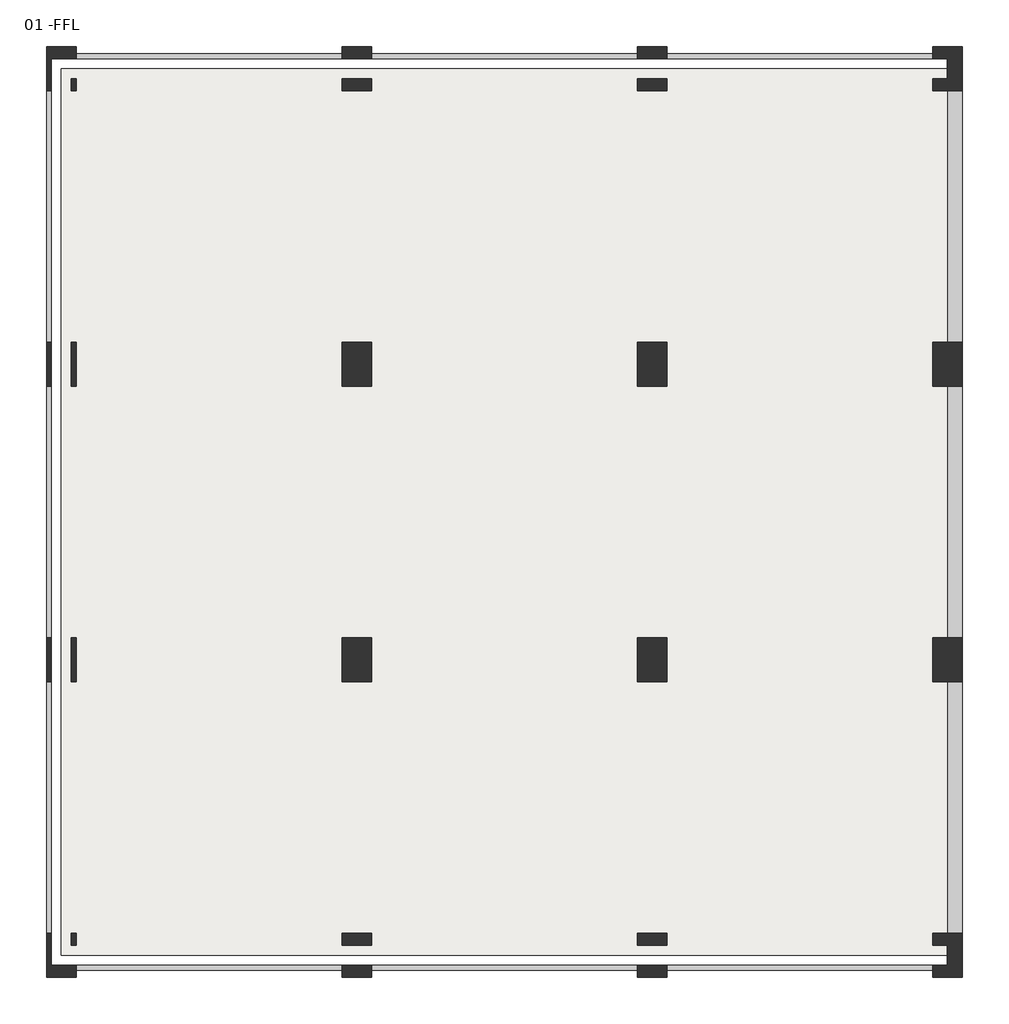
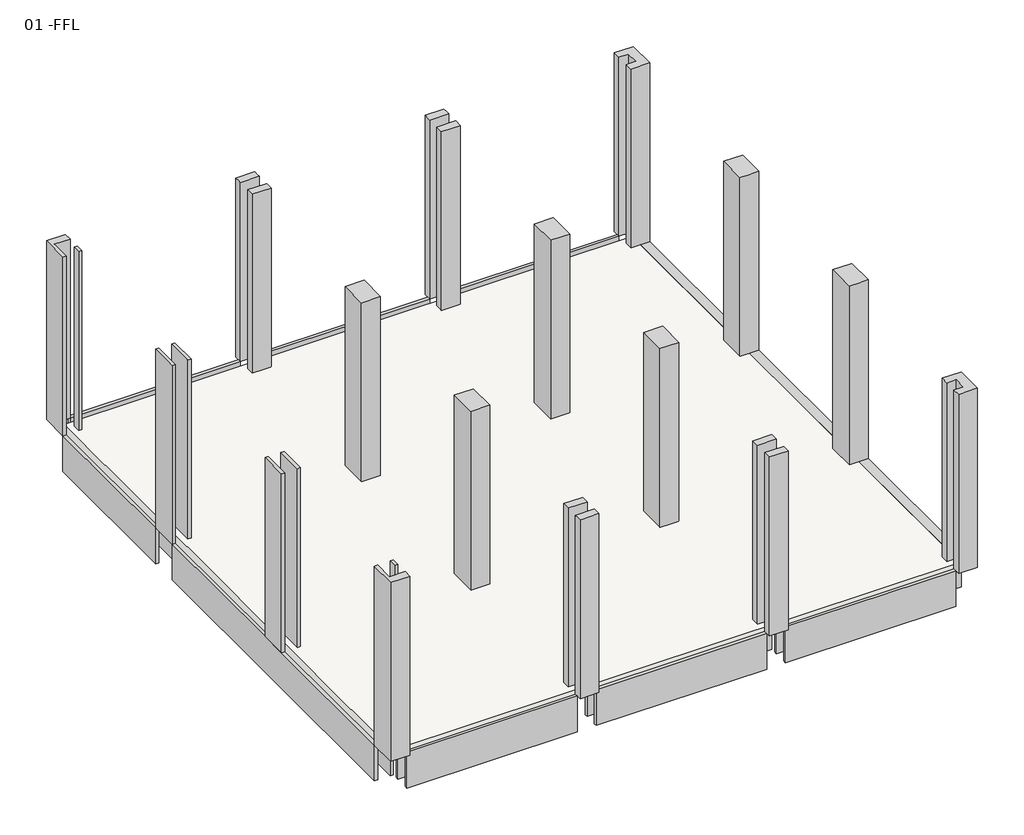
# One storey: 16 columns, 6 beams, 1 slab.
"""IFC4 building model written with IfcOpenShell, lengths in millimetres."""

from ifc_helpers import new_model, si_unit, frame, origin, place, context, project, spatial, polyline, outline, extrude, faceted_brep, element, save

model = new_model("IFC4")

# Units and contexts
model_context = context("Model", 3, world=origin())
ifc_project = project(units=[si_unit("LENGTHUNIT", "METRE", prefix="MILLI")], contexts=[model_context])

# Site, building, storey
site = spatial("IfcSite", under=ifc_project)
building = spatial("IfcBuilding", under=site)
storey = spatial("IfcBuildingStorey", under=building, Name="01 -FFL", Elevation=3048.0)

# Beams
placement = place(None, origin())
element("IfcBeam", 1, ObjectType="Concrete-Rectangular Beam : 12 x 24", at=placement, inside=storey, context=model_context, shape_type="SweptSolid", body=[
    extrude(outline(polyline([(-15593.7609662, 12775.9972109), (-12850.5609662, 12775.9972109), (-12850.5609662, 12725.1972109), (-15593.7609662, 12725.1972109), (-15593.7609662, 12775.9972109)])), frame((0.0, 0.0, 2438.4), z_axis=(0.0, 0.0, 1.0), x_axis=(1.0, 0.0, 0.0)), (0.0, 0.0, 1.0), 609.6),
    extrude(outline(polyline([(-12850.5609662, 12471.1972109), (-15593.7609662, 12471.1972109), (-15593.7609662, 12521.9972109), (-12850.5609662, 12521.9972109), (-12850.5609662, 12471.1972109)])), frame((0.0, 0.0, 2438.4), z_axis=(0.0, 0.0, 1.0), x_axis=(1.0, 0.0, 0.0)), (0.0, 0.0, 1.0), 457.2),
    extrude(outline(polyline([(-18946.5609662, 12471.1972109), (-21689.7609662, 12471.1972109), (-21689.7609662, 12521.9972109), (-18946.5609662, 12521.9972109), (-18946.5609662, 12471.1972109)])), frame((0.0, 0.0, 2438.4), z_axis=(0.0, 0.0, 1.0), x_axis=(1.0, 0.0, 0.0)), (0.0, 0.0, 1.0), 457.2),
    extrude(outline(polyline([(-15898.5609662, 12471.1972109), (-18641.7609662, 12471.1972109), (-18641.7609662, 12521.9972109), (-15898.5609662, 12521.9972109), (-15898.5609662, 12471.1972109)])), frame((0.0, 0.0, 2438.4), z_axis=(0.0, 0.0, 1.0), x_axis=(1.0, 0.0, 0.0)), (0.0, 0.0, 1.0), 457.2),
    extrude(outline(polyline([(-18641.7609662, 12775.9972109), (-15898.5609662, 12775.9972109), (-15898.5609662, 12725.1972109), (-18641.7609662, 12725.1972109), (-18641.7609662, 12775.9972109)])), frame((0.0, 0.0, 2438.4), z_axis=(0.0, 0.0, 1.0), x_axis=(1.0, 0.0, 0.0)), (0.0, 0.0, 1.0), 609.6),
    extrude(outline(polyline([(-21689.7609662, 12775.9972109), (-18946.5609662, 12775.9972109), (-18946.5609662, 12725.1972109), (-21689.7609662, 12725.1972109), (-21689.7609662, 12775.9972109)])), frame((0.0, 0.0, 2438.4), z_axis=(0.0, 0.0, 1.0), x_axis=(1.0, 0.0, 0.0)), (0.0, 0.0, 1.0), 609.6),
])
element("IfcBeam", 2, ObjectType="Concrete-Rectangular Beam : 12 x 24", at=placement, inside=storey, context=model_context, shape_type="SweptSolid", body=[
    extrude(outline(polyline([(2438.4, -12850.5609662), (2438.4, -12545.7609662), (3048.0, -12545.7609662), (3048.0, -12698.1609662), (2895.6, -12698.1609662), (2895.6, -12850.5609662), (2438.4, -12850.5609662)])), frame((0.0, 3708.1972109, 0.0), z_axis=(0.0, 1.0, 0.0), x_axis=(0.0, 0.0, 1.0)), (0.0, 0.0, 1.0), 2590.8),
    extrude(outline(polyline([(2438.4, -12850.5609662), (2438.4, -12545.7609662), (3048.0, -12545.7609662), (3048.0, -12698.1609662), (2895.6, -12698.1609662), (2895.6, -12850.5609662), (2438.4, -12850.5609662)])), frame((0.0, 9804.1972109, 0.0), z_axis=(0.0, 1.0, 0.0), x_axis=(0.0, 0.0, 1.0)), (0.0, 0.0, 1.0), 2590.8),
    extrude(outline(polyline([(2438.4, -12850.5609662), (2438.4, -12545.7609662), (3048.0, -12545.7609662), (3048.0, -12698.1609662), (2895.6, -12698.1609662), (2895.6, -12850.5609662), (2438.4, -12850.5609662)])), frame((0.0, 6756.1972109, 0.0), z_axis=(0.0, 1.0, 0.0), x_axis=(0.0, 0.0, 1.0)), (0.0, 0.0, 1.0), 2590.8),
])
element("IfcBeam", 3, ObjectType="Concrete-Rectangular Beam : 12 x 24", at=placement, inside=storey, context=model_context, shape_type="SweptSolid", body=[
    extrude(outline(polyline([(-18946.5609662, 3327.1972109), (-21689.7609662, 3327.1972109), (-21689.7609662, 3377.9972109), (-18946.5609662, 3377.9972109), (-18946.5609662, 3327.1972109)])), frame((0.0, 0.0, 2438.4), z_axis=(0.0, 0.0, 1.0), x_axis=(1.0, 0.0, 0.0)), (0.0, 0.0, 1.0), 609.6),
    extrude(outline(polyline([(-21689.7609662, 3631.9972109), (-18946.5609662, 3631.9972109), (-18946.5609662, 3581.1972109), (-21689.7609662, 3581.1972109), (-21689.7609662, 3631.9972109)])), frame((0.0, 0.0, 2438.4), z_axis=(0.0, 0.0, 1.0), x_axis=(1.0, 0.0, 0.0)), (0.0, 0.0, 1.0), 457.2),
    extrude(outline(polyline([(-12850.5609662, 3327.1972109), (-15593.7609662, 3327.1972109), (-15593.7609662, 3377.9972109), (-12850.5609662, 3377.9972109), (-12850.5609662, 3327.1972109)])), frame((0.0, 0.0, 2438.4), z_axis=(0.0, 0.0, 1.0), x_axis=(1.0, 0.0, 0.0)), (0.0, 0.0, 1.0), 609.6),
    extrude(outline(polyline([(-18641.7609662, 3631.9972109), (-15898.5609662, 3631.9972109), (-15898.5609662, 3581.1972109), (-18641.7609662, 3581.1972109), (-18641.7609662, 3631.9972109)])), frame((0.0, 0.0, 2438.4), z_axis=(0.0, 0.0, 1.0), x_axis=(1.0, 0.0, 0.0)), (0.0, 0.0, 1.0), 457.2),
    extrude(outline(polyline([(-15898.5609662, 3327.1972109), (-18641.7609662, 3327.1972109), (-18641.7609662, 3377.9972109), (-15898.5609662, 3377.9972109), (-15898.5609662, 3327.1972109)])), frame((0.0, 0.0, 2438.4), z_axis=(0.0, 0.0, 1.0), x_axis=(1.0, 0.0, 0.0)), (0.0, 0.0, 1.0), 609.6),
    extrude(outline(polyline([(-15593.7609662, 3631.9972109), (-12850.5609662, 3631.9972109), (-12850.5609662, 3581.1972109), (-15593.7609662, 3581.1972109), (-15593.7609662, 3631.9972109)])), frame((0.0, 0.0, 2438.4), z_axis=(0.0, 0.0, 1.0), x_axis=(1.0, 0.0, 0.0)), (0.0, 0.0, 1.0), 457.2),
])
element("IfcBeam", 4, ObjectType="Concrete-Rectangular Beam : 12 x 24", at=placement, inside=storey, context=model_context, shape_type="Brep", body=[
    faceted_brep([(-21994.5609662, 12394.9972109, 3048.0), (-21994.5609662, 9804.1972109, 3048.0), (-21943.7609662, 9804.1972109, 3048.0), (-21943.7609662, 12394.9972109, 3048.0), (-21994.5609662, 12394.9972109, 2438.4), (-21994.5609662, 9804.1972109, 2438.4), (-21943.7609662, 12394.9972109, 2438.4), (-21943.7609662, 9804.1972109, 2438.4)], [[[0, 1, 2, 3]], [[0, 4, 5, 1]], [[4, 0, 3, 6]], [[3, 2, 7, 6]], [[5, 4, 6, 7]], [[1, 5, 7, 2]]]),
    faceted_brep([(-21689.7609662, 9804.1972109, 2438.4), (-21689.7609662, 12394.9972109, 2438.4), (-21689.7609662, 12394.9972109, 2895.6), (-21689.7609662, 9804.1972109, 2895.6), (-21740.5609662, 9804.1972109, 2438.4), (-21740.5609662, 12394.9972109, 2438.4), (-21740.5609662, 9804.1972109, 2895.6), (-21740.5609662, 12394.9972109, 2895.6)], [[[0, 1, 2, 3]], [[1, 0, 4, 5]], [[0, 3, 6, 4]], [[3, 2, 7, 6]], [[2, 1, 5, 7]], [[5, 4, 6, 7]]]),
    faceted_brep([(-21689.7609662, 3708.1972109, 2438.4), (-21689.7609662, 3708.1972109, 2895.6), (-21740.5609662, 3708.1972109, 2895.6), (-21740.5609662, 3708.1972109, 2438.4), (-21689.7609662, 9346.9972109, 2895.6), (-21689.7609662, 9346.9972109, 2438.4), (-21740.5609662, 9346.9972109, 2438.4), (-21740.5609662, 9346.9972109, 2895.6)], [[[0, 1, 2, 3]], [[4, 5, 6, 7]], [[0, 5, 4, 1]], [[5, 0, 3, 6]], [[1, 4, 7, 2]], [[3, 2, 7, 6]]]),
    faceted_brep([(-21994.5609662, 9346.9972109, 3048.0), (-21994.5609662, 6756.1972109, 3048.0), (-21994.5609662, 6298.9972109, 3048.0), (-21994.5609662, 3708.1972109, 3048.0), (-21943.7609662, 3708.1972109, 3048.0), (-21943.7609662, 6298.9972109, 3048.0), (-21943.7609662, 6756.1972109, 3048.0), (-21943.7609662, 9346.9972109, 3048.0), (-21994.5609662, 3708.1972109, 2438.4), (-21994.5609662, 9346.9972109, 2438.4), (-21943.7609662, 3708.1972109, 2438.4), (-21943.7609662, 9346.9972109, 2438.4)], [[[0, 1, 2, 3, 4, 5, 6, 7]], [[8, 3, 2, 1, 0, 9]], [[3, 8, 10, 4]], [[9, 0, 7, 11]], [[8, 9, 11, 10]], [[4, 10, 11, 7, 6, 5]]]),
])
element("IfcBeam", 5, ObjectType="Concrete-Rectangular Beam : 12 x 24", at=placement, inside=storey, context=model_context, shape_type="SweptSolid", body=[
    extrude(outline(polyline([(-12850.5609662, 9727.9972109), (-12850.5609662, 9423.1972109), (-15593.7609662, 9423.1972109), (-15593.7609662, 9727.9972109), (-12850.5609662, 9727.9972109)])), frame((0.0, 0.0, 2438.4), z_axis=(0.0, 0.0, 1.0), x_axis=(1.0, 0.0, 0.0)), (0.0, 0.0, 1.0), 457.2),
    extrude(outline(polyline([(-21689.7609662, 9423.1972109), (-21689.7609662, 9727.9972109), (-15898.5609662, 9727.9972109), (-15898.5609662, 9423.1972109), (-21689.7609662, 9423.1972109)])), frame((0.0, 0.0, 2438.4), z_axis=(0.0, 0.0, 1.0), x_axis=(1.0, 0.0, 0.0)), (0.0, 0.0, 1.0), 457.2),
])
element("IfcBeam", 6, ObjectType="Concrete-Rectangular Beam : 12 x 24", at=placement, inside=storey, context=model_context, shape_type="SweptSolid", body=[
    extrude(outline(polyline([(-15593.7609662, 3708.1972109), (-15898.5609662, 3708.1972109), (-15898.5609662, 6298.9972109), (-15593.7609662, 6298.9972109), (-15593.7609662, 3708.1972109)])), frame((0.0, 0.0, 2438.4), z_axis=(0.0, 0.0, 1.0), x_axis=(1.0, 0.0, 0.0)), (0.0, 0.0, 1.0), 457.2),
    extrude(outline(polyline([(-15898.5609662, 12394.9972109), (-15593.7609662, 12394.9972109), (-15593.7609662, 9804.1972109), (-15898.5609662, 9804.1972109), (-15898.5609662, 12394.9972109)])), frame((0.0, 0.0, 2438.4), z_axis=(0.0, 0.0, 1.0), x_axis=(1.0, 0.0, 0.0)), (0.0, 0.0, 1.0), 457.2),
    extrude(outline(polyline([(-15898.5609662, 9346.9972109), (-15593.7609662, 9346.9972109), (-15593.7609662, 6756.1972109), (-15898.5609662, 6756.1972109), (-15898.5609662, 9346.9972109)])), frame((0.0, 0.0, 2438.4), z_axis=(0.0, 0.0, 1.0), x_axis=(1.0, 0.0, 0.0)), (0.0, 0.0, 1.0), 457.2),
])

# Columns
element("IfcColumn", 7, ObjectType="Concrete-Rectangular-Column : 12 x 18", at=placement, inside=storey, context=model_context, shape_type="SweptSolid", body=[
    extrude(outline(polyline([(-21689.7609662, 12521.9972109), (-21689.7609662, 12394.9972109), (-21740.5609662, 12394.9972109), (-21740.5609662, 12521.9972109), (-21689.7609662, 12521.9972109)])), frame((0.0, 0.0, 3048.0), z_axis=(0.0, 0.0, 1.0), x_axis=(1.0, 0.0, 0.0)), (0.0, 0.0, 1.0), 3048.0),
    extrude(outline(polyline([(-21994.5609662, 12394.9972109), (-21994.5609662, 12852.1972109), (-21689.7609662, 12852.1972109), (-21689.7609662, 12725.1972109), (-21943.7609662, 12725.1972109), (-21943.7609662, 12394.9972109), (-21994.5609662, 12394.9972109)])), frame((0.0, 0.0, 3048.0), z_axis=(0.0, 0.0, 1.0), x_axis=(1.0, 0.0, 0.0)), (0.0, 0.0, 1.0), 3048.0),
])
element("IfcColumn", 8, ObjectType="Concrete-Rectangular-Column : 12 x 18", at=placement, inside=storey, context=model_context, shape_type="Brep", body=[
    faceted_brep([(-21689.7609662, 9804.1972109, 3048.0), (-21689.7609662, 9346.9972109, 3048.0), (-21740.5609662, 9346.9972109, 3048.0), (-21740.5609662, 9804.1972109, 3048.0), (-21689.7609662, 9804.1972109, 6096.0), (-21689.7609662, 9804.1972109, 5943.6), (-21689.7609662, 9804.1972109, 5486.4), (-21740.5609662, 9804.1972109, 5486.4), (-21740.5609662, 9804.1972109, 5943.6), (-21740.5609662, 9804.1972109, 6096.0), (-21689.7609662, 9346.9972109, 6096.0), (-21689.7609662, 9346.9972109, 5943.6), (-21689.7609662, 9346.9972109, 5486.4), (-21740.5609662, 9346.9972109, 6096.0), (-21740.5609662, 9346.9972109, 5943.6), (-21740.5609662, 9346.9972109, 5486.4)], [[[0, 1, 2, 3]], [[4, 5, 6, 0, 3, 7, 8, 9]], [[1, 0, 6, 5, 4, 10, 11, 12]], [[1, 12, 11, 10, 13, 14, 15, 2]], [[3, 2, 15, 14, 13, 9, 8, 7]], [[10, 4, 9, 13]]]),
    faceted_brep([(-21994.5609662, 9804.1972109, 3048.0), (-21994.5609662, 9346.9972109, 3048.0), (-21994.5609662, 9346.9972109, 5486.4), (-21994.5609662, 9346.9972109, 6096.0), (-21994.5609662, 9804.1972109, 6096.0), (-21994.5609662, 9804.1972109, 5486.4), (-21943.7609662, 9346.9972109, 6096.0), (-21943.7609662, 9804.1972109, 6096.0), (-21943.7609662, 9346.9972109, 3048.0), (-21943.7609662, 9804.1972109, 3048.0), (-21943.7609662, 9804.1972109, 5486.4), (-21943.7609662, 9346.9972109, 5486.4)], [[[0, 1, 2, 3, 4, 5]], [[4, 3, 6, 7]], [[8, 9, 10, 7, 6, 11]], [[1, 0, 9, 8]], [[0, 5, 4, 7, 10, 9]], [[3, 2, 1, 8, 11, 6]]]),
])
element("IfcColumn", 9, ObjectType="Concrete-Rectangular-Column : 12 x 18", at=placement, inside=storey, context=model_context, shape_type="Brep", body=[
    faceted_brep([(-21689.7609662, 6756.1972109, 3048.0), (-21689.7609662, 6298.9972109, 3048.0), (-21740.5609662, 6298.9972109, 3048.0), (-21740.5609662, 6756.1972109, 3048.0), (-21689.7609662, 6756.1972109, 6096.0), (-21689.7609662, 6756.1972109, 5943.6), (-21689.7609662, 6756.1972109, 5486.4), (-21740.5609662, 6756.1972109, 5486.4), (-21740.5609662, 6756.1972109, 5943.6), (-21740.5609662, 6756.1972109, 6096.0), (-21689.7609662, 6298.9972109, 6096.0), (-21689.7609662, 6298.9972109, 5943.6), (-21689.7609662, 6298.9972109, 5486.4), (-21740.5609662, 6298.9972109, 6096.0), (-21740.5609662, 6298.9972109, 5943.6), (-21740.5609662, 6298.9972109, 5486.4)], [[[0, 1, 2, 3]], [[4, 5, 6, 0, 3, 7, 8, 9]], [[1, 0, 6, 5, 4, 10, 11, 12]], [[1, 12, 11, 10, 13, 14, 15, 2]], [[3, 2, 15, 14, 13, 9, 8, 7]], [[10, 4, 9, 13]]]),
    faceted_brep([(-21994.5609662, 6756.1972109, 3048.0), (-21994.5609662, 6298.9972109, 3048.0), (-21994.5609662, 6298.9972109, 5486.4), (-21994.5609662, 6298.9972109, 6096.0), (-21994.5609662, 6756.1972109, 6096.0), (-21994.5609662, 6756.1972109, 5486.4), (-21943.7609662, 6298.9972109, 6096.0), (-21943.7609662, 6756.1972109, 6096.0), (-21943.7609662, 6298.9972109, 3048.0), (-21943.7609662, 6756.1972109, 3048.0), (-21943.7609662, 6756.1972109, 5486.4), (-21943.7609662, 6298.9972109, 5486.4)], [[[0, 1, 2, 3, 4, 5]], [[4, 3, 6, 7]], [[8, 9, 10, 7, 6, 11]], [[1, 0, 9, 8]], [[0, 5, 4, 7, 10, 9]], [[3, 2, 1, 8, 11, 6]]]),
])
element("IfcColumn", 10, ObjectType="Concrete-Rectangular-Column : 12 x 18", at=placement, inside=storey, context=model_context, shape_type="SweptSolid", body=[
    extrude(outline(polyline([(-21740.5609662, 3708.1972109), (-21689.7609662, 3708.1972109), (-21689.7609662, 3581.1972109), (-21740.5609662, 3581.1972109), (-21740.5609662, 3708.1972109)])), frame((0.0, 0.0, 3048.0), z_axis=(0.0, 0.0, 1.0), x_axis=(1.0, 0.0, 0.0)), (0.0, 0.0, 1.0), 3048.0),
    extrude(outline(polyline([(-21994.5609662, 3250.9972109), (-21994.5609662, 3708.1972109), (-21943.7609662, 3708.1972109), (-21943.7609662, 3377.9972109), (-21689.7609662, 3377.9972109), (-21689.7609662, 3250.9972109), (-21994.5609662, 3250.9972109)])), frame((0.0, 0.0, 3048.0), z_axis=(0.0, 0.0, 1.0), x_axis=(1.0, 0.0, 0.0)), (0.0, 0.0, 1.0), 3048.0),
])
element("IfcColumn", 11, ObjectType="Concrete-Rectangular-Column : 12 x 18", at=placement, inside=storey, context=model_context, shape_type="Brep", body=[
    faceted_brep([(-18641.7609662, 12394.9972109, 3048.0), (-18946.5609662, 12394.9972109, 3048.0), (-18946.5609662, 12521.9972109, 3048.0), (-18641.7609662, 12521.9972109, 3048.0), (-18641.7609662, 12394.9972109, 6096.0), (-18641.7609662, 12521.9972109, 5486.4), (-18641.7609662, 12521.9972109, 5943.6), (-18641.7609662, 12521.9972109, 6096.0), (-18946.5609662, 12394.9972109, 6096.0), (-18946.5609662, 12521.9972109, 5486.4), (-18946.5609662, 12521.9972109, 5943.6), (-18946.5609662, 12521.9972109, 6096.0)], [[[0, 1, 2, 3]], [[4, 0, 3, 5, 6, 7]], [[1, 0, 4, 8]], [[3, 2, 9, 10, 11, 7, 6, 5]], [[1, 8, 11, 10, 9, 2]], [[8, 4, 7, 11]]]),
    faceted_brep([(-18946.5609662, 12852.1972109, 6096.0), (-18946.5609662, 12852.1972109, 3048.0), (-18946.5609662, 12725.1972109, 3048.0), (-18946.5609662, 12725.1972109, 5486.4), (-18946.5609662, 12725.1972109, 6096.0), (-18946.5609662, 12775.9972109, 6096.0), (-18641.7609662, 12852.1972109, 3048.0), (-18641.7609662, 12852.1972109, 6096.0), (-18641.7609662, 12725.1972109, 6096.0), (-18641.7609662, 12775.9972109, 6096.0), (-18641.7609662, 12725.1972109, 3048.0), (-18641.7609662, 12725.1972109, 5486.4)], [[[0, 1, 2, 3, 4, 5]], [[6, 1, 0, 7]], [[7, 0, 5, 4, 8, 9]], [[2, 10, 11, 8, 4, 3]], [[1, 6, 10, 2]], [[6, 7, 9, 8, 11, 10]]]),
])
element("IfcColumn", 12, ObjectType="Concrete-Rectangular-Column : 12 x 18", at=placement, inside=storey, context=model_context, shape_type="Brep", body=[
    faceted_brep([(-18946.5609662, 9346.9972109, 3048.0), (-18946.5609662, 9804.1972109, 3048.0), (-18641.7609662, 9804.1972109, 3048.0), (-18641.7609662, 9346.9972109, 3048.0), (-18946.5609662, 9346.9972109, 6096.0), (-18946.5609662, 9804.1972109, 6096.0), (-18946.5609662, 9804.1972109, 5943.6), (-18946.5609662, 9804.1972109, 5486.4), (-18946.5609662, 9346.9972109, 5486.4), (-18946.5609662, 9346.9972109, 5943.6), (-18641.7609662, 9804.1972109, 6096.0), (-18641.7609662, 9804.1972109, 5943.6), (-18641.7609662, 9804.1972109, 5486.4), (-18641.7609662, 9346.9972109, 6096.0), (-18641.7609662, 9346.9972109, 5943.6), (-18641.7609662, 9346.9972109, 5486.4)], [[[0, 1, 2, 3]], [[4, 5, 6, 7, 1, 0, 8, 9]], [[5, 10, 11, 12, 2, 1, 7, 6]], [[10, 13, 14, 15, 3, 2, 12, 11]], [[13, 4, 9, 8, 0, 3, 15, 14]], [[4, 13, 10, 5]]]),
])
element("IfcColumn", 13, ObjectType="Concrete-Rectangular-Column : 12 x 18", at=placement, inside=storey, context=model_context, shape_type="Brep", body=[
    faceted_brep([(-18946.5609662, 6298.9972109, 3048.0), (-18946.5609662, 6756.1972109, 3048.0), (-18641.7609662, 6756.1972109, 3048.0), (-18641.7609662, 6298.9972109, 3048.0), (-18946.5609662, 6298.9972109, 6096.0), (-18946.5609662, 6756.1972109, 6096.0), (-18946.5609662, 6756.1972109, 5943.6), (-18946.5609662, 6756.1972109, 5486.4), (-18946.5609662, 6298.9972109, 5486.4), (-18946.5609662, 6298.9972109, 5943.6), (-18641.7609662, 6756.1972109, 6096.0), (-18641.7609662, 6756.1972109, 5943.6), (-18641.7609662, 6756.1972109, 5486.4), (-18641.7609662, 6298.9972109, 6096.0), (-18641.7609662, 6298.9972109, 5943.6), (-18641.7609662, 6298.9972109, 5486.4)], [[[0, 1, 2, 3]], [[4, 5, 6, 7, 1, 0, 8, 9]], [[5, 10, 11, 12, 2, 1, 7, 6]], [[10, 13, 14, 15, 3, 2, 12, 11]], [[13, 4, 9, 8, 0, 3, 15, 14]], [[4, 13, 10, 5]]]),
])
element("IfcColumn", 14, ObjectType="Concrete-Rectangular-Column : 12 x 18", at=placement, inside=storey, context=model_context, shape_type="Brep", body=[
    faceted_brep([(-18641.7609662, 3250.9972109, 3048.0), (-18946.5609662, 3250.9972109, 3048.0), (-18946.5609662, 3377.9972109, 3048.0), (-18641.7609662, 3377.9972109, 3048.0), (-18641.7609662, 3250.9972109, 6096.0), (-18641.7609662, 3377.9972109, 5486.4), (-18641.7609662, 3377.9972109, 6096.0), (-18641.7609662, 3327.1972109, 6096.0), (-18946.5609662, 3250.9972109, 6096.0), (-18946.5609662, 3377.9972109, 5486.4), (-18946.5609662, 3377.9972109, 6096.0), (-18946.5609662, 3327.1972109, 6096.0)], [[[0, 1, 2, 3]], [[4, 0, 3, 5, 6, 7]], [[1, 0, 4, 8]], [[3, 2, 9, 10, 6, 5]], [[1, 8, 11, 10, 9, 2]], [[8, 4, 7, 6, 10, 11]]]),
    faceted_brep([(-18946.5609662, 3708.1972109, 6096.0), (-18946.5609662, 3708.1972109, 3048.0), (-18946.5609662, 3581.1972109, 3048.0), (-18946.5609662, 3581.1972109, 5486.4), (-18946.5609662, 3581.1972109, 5943.6), (-18946.5609662, 3581.1972109, 6096.0), (-18641.7609662, 3708.1972109, 3048.0), (-18641.7609662, 3708.1972109, 6096.0), (-18641.7609662, 3581.1972109, 6096.0), (-18641.7609662, 3581.1972109, 3048.0), (-18641.7609662, 3581.1972109, 5486.4), (-18641.7609662, 3581.1972109, 5943.6)], [[[0, 1, 2, 3, 4, 5]], [[6, 1, 0, 7]], [[7, 0, 5, 8]], [[2, 9, 10, 11, 8, 5, 4, 3]], [[1, 6, 9, 2]], [[6, 7, 8, 11, 10, 9]]]),
])
element("IfcColumn", 15, ObjectType="Concrete-Rectangular-Column : 12 x 18", at=placement, inside=storey, context=model_context, shape_type="Brep", body=[
    faceted_brep([(-15593.7609662, 12394.9972109, 3048.0), (-15898.5609662, 12394.9972109, 3048.0), (-15898.5609662, 12521.9972109, 3048.0), (-15593.7609662, 12521.9972109, 3048.0), (-15593.7609662, 12394.9972109, 6096.0), (-15593.7609662, 12521.9972109, 5486.4), (-15593.7609662, 12521.9972109, 5943.6), (-15593.7609662, 12521.9972109, 6096.0), (-15898.5609662, 12394.9972109, 6096.0), (-15898.5609662, 12521.9972109, 5486.4), (-15898.5609662, 12521.9972109, 5943.6), (-15898.5609662, 12521.9972109, 6096.0)], [[[0, 1, 2, 3]], [[4, 0, 3, 5, 6, 7]], [[1, 0, 4, 8]], [[3, 2, 9, 10, 11, 7, 6, 5]], [[1, 8, 11, 10, 9, 2]], [[8, 4, 7, 11]]]),
    faceted_brep([(-15898.5609662, 12852.1972109, 6096.0), (-15898.5609662, 12852.1972109, 3048.0), (-15898.5609662, 12725.1972109, 3048.0), (-15898.5609662, 12725.1972109, 5486.4), (-15898.5609662, 12725.1972109, 6096.0), (-15898.5609662, 12775.9972109, 6096.0), (-15593.7609662, 12852.1972109, 3048.0), (-15593.7609662, 12852.1972109, 6096.0), (-15593.7609662, 12725.1972109, 6096.0), (-15593.7609662, 12775.9972109, 6096.0), (-15593.7609662, 12725.1972109, 3048.0), (-15593.7609662, 12725.1972109, 5486.4)], [[[0, 1, 2, 3, 4, 5]], [[6, 1, 0, 7]], [[7, 0, 5, 4, 8, 9]], [[2, 10, 11, 8, 4, 3]], [[1, 6, 10, 2]], [[6, 7, 9, 8, 11, 10]]]),
])
element("IfcColumn", 16, ObjectType="Concrete-Rectangular-Column : 12 x 18", at=placement, inside=storey, context=model_context, shape_type="Brep", body=[
    faceted_brep([(-15898.5609662, 9346.9972109, 3048.0), (-15898.5609662, 9804.1972109, 3048.0), (-15593.7609662, 9804.1972109, 3048.0), (-15593.7609662, 9346.9972109, 3048.0), (-15898.5609662, 9346.9972109, 6096.0), (-15898.5609662, 9804.1972109, 6096.0), (-15898.5609662, 9804.1972109, 5943.6), (-15898.5609662, 9804.1972109, 5486.4), (-15898.5609662, 9346.9972109, 5486.4), (-15898.5609662, 9346.9972109, 5943.6), (-15593.7609662, 9804.1972109, 6096.0), (-15593.7609662, 9804.1972109, 5943.6), (-15593.7609662, 9804.1972109, 5486.4), (-15593.7609662, 9346.9972109, 6096.0), (-15593.7609662, 9346.9972109, 5943.6), (-15593.7609662, 9346.9972109, 5486.4)], [[[0, 1, 2, 3]], [[4, 5, 6, 7, 1, 0, 8, 9]], [[5, 10, 11, 12, 2, 1, 7, 6]], [[10, 13, 14, 15, 3, 2, 12, 11]], [[13, 4, 9, 8, 0, 3, 15, 14]], [[4, 13, 10, 5]]]),
])
element("IfcColumn", 17, ObjectType="Concrete-Rectangular-Column : 12 x 18", at=placement, inside=storey, context=model_context, shape_type="Brep", body=[
    faceted_brep([(-15898.5609662, 6298.9972109, 3048.0), (-15898.5609662, 6756.1972109, 3048.0), (-15593.7609662, 6756.1972109, 3048.0), (-15593.7609662, 6298.9972109, 3048.0), (-15898.5609662, 6298.9972109, 6096.0), (-15898.5609662, 6756.1972109, 6096.0), (-15898.5609662, 6756.1972109, 5943.6), (-15898.5609662, 6756.1972109, 5486.4), (-15898.5609662, 6298.9972109, 5486.4), (-15898.5609662, 6298.9972109, 5943.6), (-15593.7609662, 6756.1972109, 6096.0), (-15593.7609662, 6756.1972109, 5943.6), (-15593.7609662, 6756.1972109, 5486.4), (-15593.7609662, 6298.9972109, 6096.0), (-15593.7609662, 6298.9972109, 5943.6), (-15593.7609662, 6298.9972109, 5486.4)], [[[0, 1, 2, 3]], [[4, 5, 6, 7, 1, 0, 8, 9]], [[5, 10, 11, 12, 2, 1, 7, 6]], [[10, 13, 14, 15, 3, 2, 12, 11]], [[13, 4, 9, 8, 0, 3, 15, 14]], [[4, 13, 10, 5]]]),
])
element("IfcColumn", 18, ObjectType="Concrete-Rectangular-Column : 12 x 18", at=placement, inside=storey, context=model_context, shape_type="Brep", body=[
    faceted_brep([(-15593.7609662, 3250.9972109, 3048.0), (-15898.5609662, 3250.9972109, 3048.0), (-15898.5609662, 3377.9972109, 3048.0), (-15593.7609662, 3377.9972109, 3048.0), (-15593.7609662, 3250.9972109, 6096.0), (-15593.7609662, 3377.9972109, 5486.4), (-15593.7609662, 3377.9972109, 6096.0), (-15593.7609662, 3327.1972109, 6096.0), (-15898.5609662, 3250.9972109, 6096.0), (-15898.5609662, 3377.9972109, 5486.4), (-15898.5609662, 3377.9972109, 6096.0), (-15898.5609662, 3327.1972109, 6096.0)], [[[0, 1, 2, 3]], [[4, 0, 3, 5, 6, 7]], [[1, 0, 4, 8]], [[3, 2, 9, 10, 6, 5]], [[1, 8, 11, 10, 9, 2]], [[8, 4, 7, 6, 10, 11]]]),
    faceted_brep([(-15898.5609662, 3708.1972109, 6096.0), (-15898.5609662, 3708.1972109, 3048.0), (-15898.5609662, 3581.1972109, 3048.0), (-15898.5609662, 3581.1972109, 5486.4), (-15898.5609662, 3581.1972109, 5943.6), (-15898.5609662, 3581.1972109, 6096.0), (-15593.7609662, 3708.1972109, 3048.0), (-15593.7609662, 3708.1972109, 6096.0), (-15593.7609662, 3581.1972109, 6096.0), (-15593.7609662, 3581.1972109, 3048.0), (-15593.7609662, 3581.1972109, 5486.4), (-15593.7609662, 3581.1972109, 5943.6)], [[[0, 1, 2, 3, 4, 5]], [[6, 1, 0, 7]], [[7, 0, 5, 8]], [[2, 9, 10, 11, 8, 5, 4, 3]], [[1, 6, 9, 2]], [[6, 7, 8, 11, 10, 9]]]),
])
element("IfcColumn", 19, ObjectType="Concrete-Rectangular-Column : 12 x 18", at=placement, inside=storey, context=model_context, shape_type="SweptSolid", body=[
    extrude(outline(polyline([(-12850.5609662, 12852.1972109), (-12545.7609662, 12852.1972109), (-12545.7609662, 12394.9972109), (-12850.5609662, 12394.9972109), (-12850.5609662, 12521.9972109), (-12698.1609662, 12521.9972109), (-12698.1609662, 12725.1972109), (-12850.5609662, 12725.1972109), (-12850.5609662, 12852.1972109)])), frame((0.0, 0.0, 3048.0), z_axis=(0.0, 0.0, 1.0), x_axis=(1.0, 0.0, 0.0)), (0.0, 0.0, 1.0), 3048.0),
])
element("IfcColumn", 20, ObjectType="Concrete-Rectangular-Column : 12 x 18", at=placement, inside=storey, context=model_context, shape_type="Brep", body=[
    faceted_brep([(-12850.5609662, 9346.9972109, 3048.0), (-12850.5609662, 9804.1972109, 3048.0), (-12545.7609662, 9804.1972109, 3048.0), (-12545.7609662, 9346.9972109, 3048.0), (-12850.5609662, 9346.9972109, 6096.0), (-12850.5609662, 9804.1972109, 6096.0), (-12850.5609662, 9804.1972109, 5943.6), (-12850.5609662, 9804.1972109, 5486.4), (-12850.5609662, 9346.9972109, 5486.4), (-12850.5609662, 9346.9972109, 5943.6), (-12698.1609662, 9804.1972109, 6096.0), (-12545.7609662, 9804.1972109, 6096.0), (-12545.7609662, 9804.1972109, 5486.4), (-12545.7609662, 9346.9972109, 6096.0), (-12545.7609662, 9346.9972109, 5486.4), (-12698.1609662, 9346.9972109, 6096.0)], [[[0, 1, 2, 3]], [[4, 5, 6, 7, 1, 0, 8, 9]], [[5, 10, 11, 12, 2, 1, 7, 6]], [[11, 13, 14, 3, 2, 12]], [[13, 15, 4, 9, 8, 0, 3, 14]], [[4, 15, 13, 11, 10, 5]]]),
])
element("IfcColumn", 21, ObjectType="Concrete-Rectangular-Column : 12 x 18", at=placement, inside=storey, context=model_context, shape_type="Brep", body=[
    faceted_brep([(-12850.5609662, 6298.9972109, 3048.0), (-12850.5609662, 6756.1972109, 3048.0), (-12545.7609662, 6756.1972109, 3048.0), (-12545.7609662, 6298.9972109, 3048.0), (-12850.5609662, 6298.9972109, 6096.0), (-12850.5609662, 6756.1972109, 6096.0), (-12850.5609662, 6756.1972109, 5943.6), (-12850.5609662, 6756.1972109, 5486.4), (-12850.5609662, 6298.9972109, 5486.4), (-12850.5609662, 6298.9972109, 5943.6), (-12698.1609662, 6756.1972109, 6096.0), (-12545.7609662, 6756.1972109, 6096.0), (-12545.7609662, 6756.1972109, 5486.4), (-12545.7609662, 6298.9972109, 6096.0), (-12545.7609662, 6298.9972109, 5486.4), (-12698.1609662, 6298.9972109, 6096.0)], [[[0, 1, 2, 3]], [[4, 5, 6, 7, 1, 0, 8, 9]], [[5, 10, 11, 12, 2, 1, 7, 6]], [[11, 13, 14, 3, 2, 12]], [[13, 15, 4, 9, 8, 0, 3, 14]], [[4, 15, 13, 11, 10, 5]]]),
])
element("IfcColumn", 22, ObjectType="Concrete-Rectangular-Column : 12 x 18", at=placement, inside=storey, context=model_context, shape_type="SweptSolid", body=[
    extrude(outline(polyline([(-12850.5609662, 3708.1972109), (-12545.7609662, 3708.1972109), (-12545.7609662, 3250.9972109), (-12850.5609662, 3250.9972109), (-12850.5609662, 3377.9972109), (-12698.1609662, 3377.9972109), (-12698.1609662, 3581.1972109), (-12850.5609662, 3581.1972109), (-12850.5609662, 3708.1972109)])), frame((0.0, 0.0, 3048.0), z_axis=(0.0, 0.0, 1.0), x_axis=(1.0, 0.0, 0.0)), (0.0, 0.0, 1.0), 3048.0),
])

# Slab
element("IfcSlab", 23, ObjectType="6\" Foundation Slab", at=placement, inside=storey, context=model_context, shape_type="Brep", body=[
    faceted_brep([(-12698.1609662, 12623.5972109, 2895.6), (-12698.1609662, 12394.9972109, 2895.6), (-12698.1609662, 9804.1972109, 2895.6), (-12698.1609662, 9346.9972109, 2895.6), (-12698.1609662, 6756.1972109, 2895.6), (-12698.1609662, 6298.9972109, 2895.6), (-12698.1609662, 3708.1972109, 2895.6), (-12698.1609662, 3479.5972109, 2895.6), (-21842.1609662, 3479.5972109, 2895.6), (-21842.1609662, 12623.5972109, 2895.6), (-12698.1609662, 12623.5972109, 3048.0), (-21842.1609662, 12623.5972109, 3048.0), (-21842.1609662, 3479.5972109, 3048.0), (-12698.1609662, 3479.5972109, 3048.0), (-12698.1609662, 3708.1972109, 3048.0), (-12698.1609662, 6298.9972109, 3048.0), (-12698.1609662, 6756.1972109, 3048.0), (-12698.1609662, 9346.9972109, 3048.0), (-12698.1609662, 9804.1972109, 3048.0), (-12698.1609662, 12394.9972109, 3048.0)], [[[0, 1, 2, 3, 4, 5, 6, 7, 8, 9]], [[10, 11, 12, 13, 14, 15, 16, 17, 18, 19]], [[7, 6, 5, 4, 3, 2, 1, 0, 10, 19, 18, 17, 16, 15, 14, 13]], [[8, 7, 13, 12]], [[9, 8, 12, 11]], [[0, 9, 11, 10]]]),
])

save(model, "model.ifc")

# Revit data of these elements
# Type "Concrete-Rectangular Beam : 12 x 24"
#   Assembly Code = "B10"
#   Length [instance default] = 5' - 0"
#   b = 1' - 0"
#   h = 2' - 0"
#   Structural Material [instance default] = Concrete, Cast-in-Place gray
# Type "Concrete-Rectangular-Column : 12 x 18"
#   Assembly Code = "B10"
#   b = 1' - 0"
#   h = 1' - 6"
#   Structural Material [instance default] = Concrete, Cast-in-Place gray
# Type "6\" Foundation Slab"
#   Layers, outside or top first: 0' - 6" "Concrete, Cast-in-Place gray" (function 1)
# Elements 1, 2, 3, 4, 5, 6 (IfcBeam, "Concrete-Rectangular Beam : 12 x 24")
#   Structural Material = Concrete, Cast-in-Place gray
#   Phase Created = New Construction
#   Materials on its faces: "Concrete, Cast-in-Place gray"
# Elements 7, 8, 9, 10, 11, 12, 13, 14, 15, 16, 17, 18, 19, 20, 21, 22 (IfcColumn, "Concrete-Rectangular-Column : 12 x 18")
#   Comments = ""
#   Structural Material = Concrete, Cast-in-Place gray
#   Phase Created = New Construction
#   Materials on its faces: "Concrete, Cast-in-Place gray"
# Element 23 (IfcSlab, "6\" Foundation Slab")
#   Height Offset From Level = 0' - 0"
#   built-in parameter 1001954 = 1
#   Phase Created = New Construction
#   Materials on its faces: "Concrete, Cast-in-Place gray"
# Materials
#   "Concrete, Cast-in-Place gray": class "Concrete", colour RGB 192 192 192, transparency 0, Description = "Cast-in-place concrete", Cost = 0
